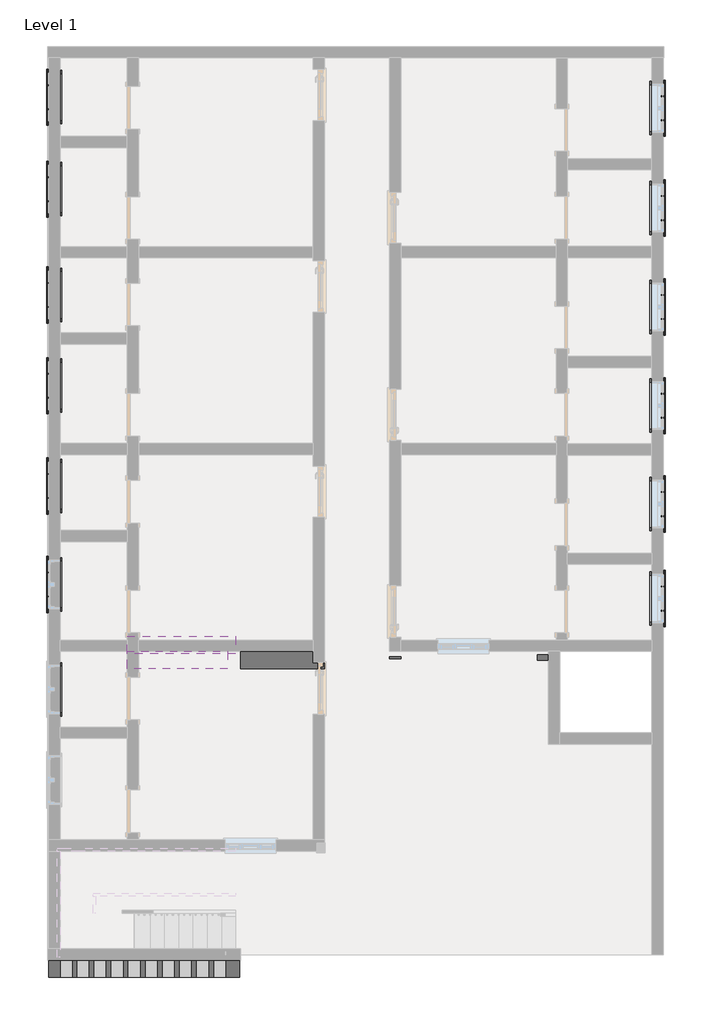
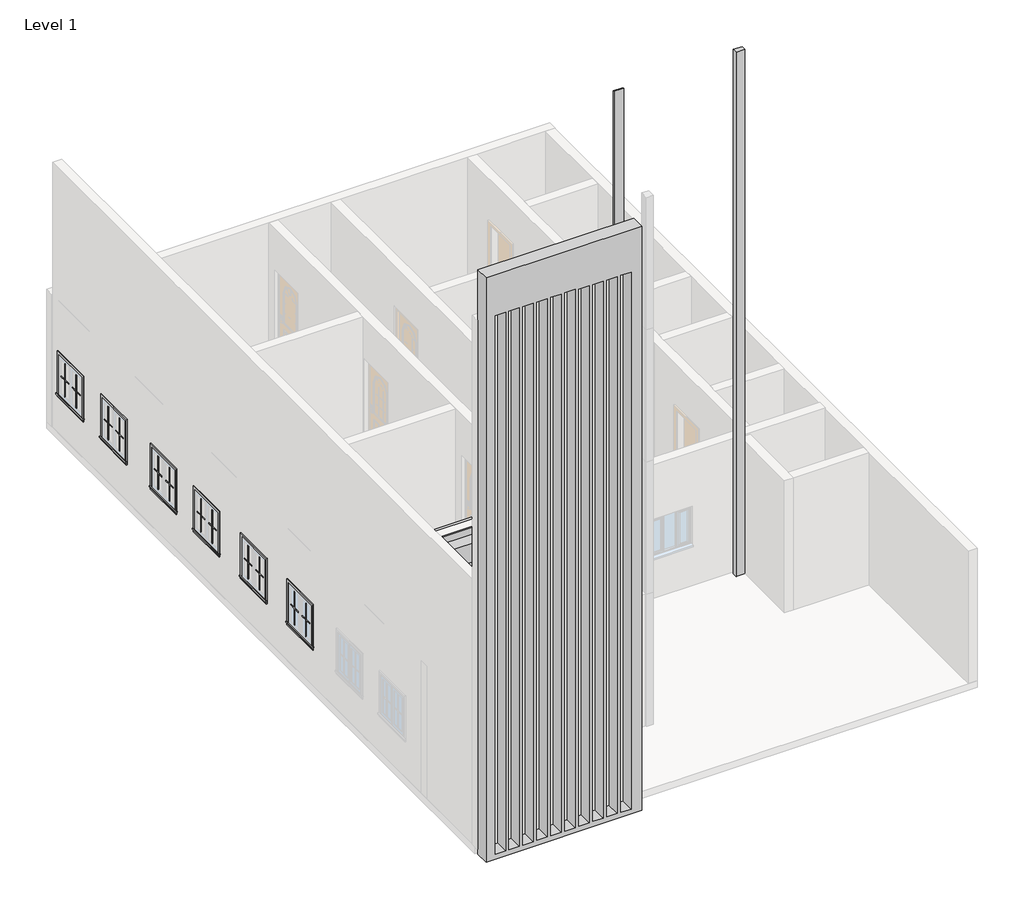
# One storey, part 4 of 4: 54 proxies.
"""IFC4 building model written with IfcOpenShell, lengths in millimetres."""

from ifc_helpers import new_model, si_unit, origin, place, context, project, spatial, transform, mapped, element, save
from components import generic_models_1_generic_models_1_2151a878, generic_models_2_generic_models_2_263b720d, generic_models_3_generic_models_3_38643fe6, generic_models_4_generic_models_4_c09d9ab6, generic_models_5_generic_models_5_710787d1, muntin_pattern_2x2_muntin_pattern_2x2_b3fe6957, muntin_pattern_2x2_muntin_pattern_2x2_3e0ecaf2, trim_window_exterior_flat_with_sill_41619996, trim_window_interior_flat_picture_frame_51c85655

model = new_model("IFC4")

# Units and contexts
model_context = context("Model", 3, world=origin())
ifc_project = project(units=[si_unit("LENGTHUNIT", "METRE", prefix="MILLI")], contexts=[model_context])

# Site, building, storey
site = spatial("IfcSite", under=ifc_project)
building = spatial("IfcBuilding", under=site)
storey = spatial("IfcBuildingStorey", under=building, Name="Level 1", Elevation=0.0)

# Proxies
placement = place(None, origin())
generic_models_1_generic_models_1_shape = generic_models_1_generic_models_1_2151a878(model_context)
element("IfcBuildingElementProxy", 1, Name="Generic Models 1 : Generic Models 1", ObjectType="Generic Models 1 : Generic Models 1", at=placement, inside=storey, context=model_context, shape_type="MappedRepresentation", body=[
    mapped(generic_models_1_generic_models_1_shape, transform((0.0, 0.0, 0.0), x_axis=(1.0, 0.0, 0.0), y_axis=(0.0, 1.0, 0.0), z_axis=(0.0, 0.0, 1.0))),
])
generic_models_2_generic_models_2_shape = generic_models_2_generic_models_2_263b720d(model_context)
element("IfcBuildingElementProxy", 2, Name="Generic Models 2 : Generic Models 2", ObjectType="Generic Models 2 : Generic Models 2", at=placement, inside=storey, context=model_context, shape_type="MappedRepresentation", body=[
    mapped(generic_models_2_generic_models_2_shape, transform((0.0, 0.0, 0.0), x_axis=(1.0, 0.0, 0.0), y_axis=(0.0, 1.0, 0.0), z_axis=(0.0, 0.0, 1.0))),
])
generic_models_3_generic_models_3_shape = generic_models_3_generic_models_3_38643fe6(model_context)
element("IfcBuildingElementProxy", 3, Name="Generic Models 3 : Generic Models 3", ObjectType="Generic Models 3 : Generic Models 3", at=placement, inside=storey, context=model_context, shape_type="MappedRepresentation", body=[
    mapped(generic_models_3_generic_models_3_shape, transform((0.0, 0.0, 0.0), x_axis=(1.0, 0.0, 0.0), y_axis=(0.0, 1.0, 0.0), z_axis=(0.0, 0.0, 1.0))),
])
generic_models_4_generic_models_4_shape = generic_models_4_generic_models_4_c09d9ab6(model_context)
element("IfcBuildingElementProxy", 4, Name="Generic Models 4 : Generic Models 4", ObjectType="Generic Models 4 : Generic Models 4", at=placement, inside=storey, context=model_context, shape_type="MappedRepresentation", body=[
    mapped(generic_models_4_generic_models_4_shape, transform((0.0, 0.0, 0.0), x_axis=(1.0, 0.0, 0.0), y_axis=(0.0, 1.0, 0.0), z_axis=(0.0, 0.0, 1.0))),
])
generic_models_5_generic_models_5_shape = generic_models_5_generic_models_5_710787d1(model_context)
element("IfcBuildingElementProxy", 5, Name="Generic Models 5 : Generic Models 5", ObjectType="Generic Models 5 : Generic Models 5", at=placement, inside=storey, context=model_context, shape_type="MappedRepresentation", body=[
    mapped(generic_models_5_generic_models_5_shape, transform((0.0, 0.0, 0.0), x_axis=(1.0, 0.0, 0.0), y_axis=(0.0, 1.0, 0.0), z_axis=(0.0, 0.0, 1.0))),
])
muntin_pattern_2x2_muntin_pattern_2x2_shape = muntin_pattern_2x2_muntin_pattern_2x2_b3fe6957(model_context)
element("IfcBuildingElementProxy", 6, Name="Muntin Pattern_2x2 : Muntin Pattern_2x2", ObjectType="Muntin Pattern_2x2 : Muntin Pattern_2x2", at=placement, inside=storey, context=model_context, shape_type="MappedRepresentation", body=[
    mapped(muntin_pattern_2x2_muntin_pattern_2x2_shape, transform((-6438.8858866, 6882.8274728, 984.25), x_axis=(0.0, 1.0, 0.0), y_axis=(-1.0, 0.0, 0.0), z_axis=(0.0, 0.0, 1.0))),
])
element("IfcBuildingElementProxy", 7, Name="Muntin Pattern_2x2 : Muntin Pattern_2x2", ObjectType="Muntin Pattern_2x2 : Muntin Pattern_2x2", at=placement, inside=storey, context=model_context, shape_type="MappedRepresentation", body=[
    mapped(muntin_pattern_2x2_muntin_pattern_2x2_shape, transform((-6438.8858866, 5244.5274728, 984.25), x_axis=(0.0, 1.0, 0.0), y_axis=(-1.0, 0.0, 0.0), z_axis=(0.0, 0.0, 1.0))),
])
element("IfcBuildingElementProxy", 8, Name="Muntin Pattern_2x2 : Muntin Pattern_2x2", ObjectType="Muntin Pattern_2x2 : Muntin Pattern_2x2", at=placement, inside=storey, context=model_context, shape_type="MappedRepresentation", body=[
    mapped(muntin_pattern_2x2_muntin_pattern_2x2_shape, transform((-6438.8858866, 3360.4810874, 984.25), x_axis=(0.0, 1.0, 0.0), y_axis=(-1.0, 0.0, 0.0), z_axis=(0.0, 0.0, 1.0))),
])
element("IfcBuildingElementProxy", 9, Name="Muntin Pattern_2x2 : Muntin Pattern_2x2", ObjectType="Muntin Pattern_2x2 : Muntin Pattern_2x2", at=placement, inside=storey, context=model_context, shape_type="MappedRepresentation", body=[
    mapped(muntin_pattern_2x2_muntin_pattern_2x2_shape, transform((-6438.8858866, 1745.426343, 984.25), x_axis=(0.0, 1.0, 0.0), y_axis=(-1.0, 0.0, 0.0), z_axis=(0.0, 0.0, 1.0))),
])
element("IfcBuildingElementProxy", 10, Name="Muntin Pattern_2x2 : Muntin Pattern_2x2", ObjectType="Muntin Pattern_2x2 : Muntin Pattern_2x2", at=placement, inside=storey, context=model_context, shape_type="MappedRepresentation", body=[
    mapped(muntin_pattern_2x2_muntin_pattern_2x2_shape, transform((-6438.8858866, -38.6725272, 984.25), x_axis=(0.0, 1.0, 0.0), y_axis=(-1.0, 0.0, 0.0), z_axis=(0.0, 0.0, 1.0))),
])
element("IfcBuildingElementProxy", 11, Name="Muntin Pattern_2x2 : Muntin Pattern_2x2", ObjectType="Muntin Pattern_2x2 : Muntin Pattern_2x2", at=placement, inside=storey, context=model_context, shape_type="MappedRepresentation", body=[
    mapped(muntin_pattern_2x2_muntin_pattern_2x2_shape, transform((-6438.8858866, -1791.2725272, 984.25), x_axis=(0.0, 1.0, 0.0), y_axis=(-1.0, 0.0, 0.0), z_axis=(0.0, 0.0, 1.0))),
])
element("IfcBuildingElementProxy", 12, Name="Muntin Pattern_2x2 : Muntin Pattern_2x2", ObjectType="Muntin Pattern_2x2 : Muntin Pattern_2x2", at=placement, inside=storey, context=model_context, shape_type="MappedRepresentation", body=[
    mapped(muntin_pattern_2x2_muntin_pattern_2x2_shape, transform((4489.4641134, -1616.6475272, 984.25), x_axis=(0.0, -1.0, 0.0), y_axis=(1.0, 0.0, 0.0), z_axis=(0.0, 0.0, 1.0))),
])
element("IfcBuildingElementProxy", 13, Name="Muntin Pattern_2x2 : Muntin Pattern_2x2", ObjectType="Muntin Pattern_2x2 : Muntin Pattern_2x2", at=placement, inside=storey, context=model_context, shape_type="MappedRepresentation", body=[
    mapped(muntin_pattern_2x2_muntin_pattern_2x2_shape, transform((4489.4641134, 66.1024728, 984.25), x_axis=(0.0, -1.0, 0.0), y_axis=(1.0, 0.0, 0.0), z_axis=(0.0, 0.0, 1.0))),
])
element("IfcBuildingElementProxy", 14, Name="Muntin Pattern_2x2 : Muntin Pattern_2x2", ObjectType="Muntin Pattern_2x2 : Muntin Pattern_2x2", at=placement, inside=storey, context=model_context, shape_type="MappedRepresentation", body=[
    mapped(muntin_pattern_2x2_muntin_pattern_2x2_shape, transform((4489.4641134, 1818.7024728, 984.25), x_axis=(0.0, -1.0, 0.0), y_axis=(1.0, 0.0, 0.0), z_axis=(0.0, 0.0, 1.0))),
])
element("IfcBuildingElementProxy", 15, Name="Muntin Pattern_2x2 : Muntin Pattern_2x2", ObjectType="Muntin Pattern_2x2 : Muntin Pattern_2x2", at=placement, inside=storey, context=model_context, shape_type="MappedRepresentation", body=[
    mapped(muntin_pattern_2x2_muntin_pattern_2x2_shape, transform((4489.4641134, 3577.6524728, 984.25), x_axis=(0.0, -1.0, 0.0), y_axis=(1.0, 0.0, 0.0), z_axis=(0.0, 0.0, 1.0))),
])
element("IfcBuildingElementProxy", 16, Name="Muntin Pattern_2x2 : Muntin Pattern_2x2", ObjectType="Muntin Pattern_2x2 : Muntin Pattern_2x2", at=placement, inside=storey, context=model_context, shape_type="MappedRepresentation", body=[
    mapped(muntin_pattern_2x2_muntin_pattern_2x2_shape, transform((4489.4641134, 5336.6024728, 984.25), x_axis=(0.0, -1.0, 0.0), y_axis=(1.0, 0.0, 0.0), z_axis=(0.0, 0.0, 1.0))),
])
element("IfcBuildingElementProxy", 17, Name="Muntin Pattern_2x2 : Muntin Pattern_2x2", ObjectType="Muntin Pattern_2x2 : Muntin Pattern_2x2", at=placement, inside=storey, context=model_context, shape_type="MappedRepresentation", body=[
    mapped(muntin_pattern_2x2_muntin_pattern_2x2_shape, transform((4489.4641134, 7114.6024728, 984.25), x_axis=(0.0, -1.0, 0.0), y_axis=(1.0, 0.0, 0.0), z_axis=(0.0, 0.0, 1.0))),
])
muntin_pattern_2x2_muntin_pattern_2x2_2_shape = muntin_pattern_2x2_muntin_pattern_2x2_3e0ecaf2(model_context)
element("IfcBuildingElementProxy", 18, Name="Muntin Pattern_2x2 : Muntin Pattern_2x2", ObjectType="Muntin Pattern_2x2 : Muntin Pattern_2x2", at=placement, inside=storey, context=model_context, shape_type="MappedRepresentation", body=[
    mapped(muntin_pattern_2x2_muntin_pattern_2x2_2_shape, transform((-6438.8858866, 7311.4524728, 984.25), x_axis=(0.0, -1.0, 0.0), y_axis=(1.0, 0.0, 0.0), z_axis=(0.0, 0.0, 1.0))),
])
element("IfcBuildingElementProxy", 19, Name="Muntin Pattern_2x2 : Muntin Pattern_2x2", ObjectType="Muntin Pattern_2x2 : Muntin Pattern_2x2", at=placement, inside=storey, context=model_context, shape_type="MappedRepresentation", body=[
    mapped(muntin_pattern_2x2_muntin_pattern_2x2_2_shape, transform((-6438.8858866, 5673.1524728, 984.25), x_axis=(0.0, -1.0, 0.0), y_axis=(1.0, 0.0, 0.0), z_axis=(0.0, 0.0, 1.0))),
])
element("IfcBuildingElementProxy", 20, Name="Muntin Pattern_2x2 : Muntin Pattern_2x2", ObjectType="Muntin Pattern_2x2 : Muntin Pattern_2x2", at=placement, inside=storey, context=model_context, shape_type="MappedRepresentation", body=[
    mapped(muntin_pattern_2x2_muntin_pattern_2x2_2_shape, transform((-6438.8858866, 3789.1060874, 984.25), x_axis=(0.0, -1.0, 0.0), y_axis=(1.0, 0.0, 0.0), z_axis=(0.0, 0.0, 1.0))),
])
element("IfcBuildingElementProxy", 21, Name="Muntin Pattern_2x2 : Muntin Pattern_2x2", ObjectType="Muntin Pattern_2x2 : Muntin Pattern_2x2", at=placement, inside=storey, context=model_context, shape_type="MappedRepresentation", body=[
    mapped(muntin_pattern_2x2_muntin_pattern_2x2_2_shape, transform((-6438.8858866, 2174.051343, 984.25), x_axis=(0.0, -1.0, 0.0), y_axis=(1.0, 0.0, 0.0), z_axis=(0.0, 0.0, 1.0))),
])
element("IfcBuildingElementProxy", 22, Name="Muntin Pattern_2x2 : Muntin Pattern_2x2", ObjectType="Muntin Pattern_2x2 : Muntin Pattern_2x2", at=placement, inside=storey, context=model_context, shape_type="MappedRepresentation", body=[
    mapped(muntin_pattern_2x2_muntin_pattern_2x2_2_shape, transform((-6438.8858866, 389.9524728, 984.25), x_axis=(0.0, -1.0, 0.0), y_axis=(1.0, 0.0, 0.0), z_axis=(0.0, 0.0, 1.0))),
])
element("IfcBuildingElementProxy", 23, Name="Muntin Pattern_2x2 : Muntin Pattern_2x2", ObjectType="Muntin Pattern_2x2 : Muntin Pattern_2x2", at=placement, inside=storey, context=model_context, shape_type="MappedRepresentation", body=[
    mapped(muntin_pattern_2x2_muntin_pattern_2x2_2_shape, transform((-6438.8858866, -1362.6475272, 984.25), x_axis=(0.0, -1.0, 0.0), y_axis=(1.0, 0.0, 0.0), z_axis=(0.0, 0.0, 1.0))),
])
element("IfcBuildingElementProxy", 24, Name="Muntin Pattern_2x2 : Muntin Pattern_2x2", ObjectType="Muntin Pattern_2x2 : Muntin Pattern_2x2", at=placement, inside=storey, context=model_context, shape_type="MappedRepresentation", body=[
    mapped(muntin_pattern_2x2_muntin_pattern_2x2_2_shape, transform((4489.4641134, -2045.2725272, 984.25), x_axis=(0.0, 1.0, 0.0), y_axis=(-1.0, 0.0, 0.0), z_axis=(0.0, 0.0, 1.0))),
])
element("IfcBuildingElementProxy", 25, Name="Muntin Pattern_2x2 : Muntin Pattern_2x2", ObjectType="Muntin Pattern_2x2 : Muntin Pattern_2x2", at=placement, inside=storey, context=model_context, shape_type="MappedRepresentation", body=[
    mapped(muntin_pattern_2x2_muntin_pattern_2x2_2_shape, transform((4489.4641134, -362.5225272, 984.25), x_axis=(0.0, 1.0, 0.0), y_axis=(-1.0, 0.0, 0.0), z_axis=(0.0, 0.0, 1.0))),
])
element("IfcBuildingElementProxy", 26, Name="Muntin Pattern_2x2 : Muntin Pattern_2x2", ObjectType="Muntin Pattern_2x2 : Muntin Pattern_2x2", at=placement, inside=storey, context=model_context, shape_type="MappedRepresentation", body=[
    mapped(muntin_pattern_2x2_muntin_pattern_2x2_2_shape, transform((4489.4641134, 1390.0774728, 984.25), x_axis=(0.0, 1.0, 0.0), y_axis=(-1.0, 0.0, 0.0), z_axis=(0.0, 0.0, 1.0))),
])
element("IfcBuildingElementProxy", 27, Name="Muntin Pattern_2x2 : Muntin Pattern_2x2", ObjectType="Muntin Pattern_2x2 : Muntin Pattern_2x2", at=placement, inside=storey, context=model_context, shape_type="MappedRepresentation", body=[
    mapped(muntin_pattern_2x2_muntin_pattern_2x2_2_shape, transform((4489.4641134, 3149.0274728, 984.25), x_axis=(0.0, 1.0, 0.0), y_axis=(-1.0, 0.0, 0.0), z_axis=(0.0, 0.0, 1.0))),
])
element("IfcBuildingElementProxy", 28, Name="Muntin Pattern_2x2 : Muntin Pattern_2x2", ObjectType="Muntin Pattern_2x2 : Muntin Pattern_2x2", at=placement, inside=storey, context=model_context, shape_type="MappedRepresentation", body=[
    mapped(muntin_pattern_2x2_muntin_pattern_2x2_2_shape, transform((4489.4641134, 4907.9774728, 984.25), x_axis=(0.0, 1.0, 0.0), y_axis=(-1.0, 0.0, 0.0), z_axis=(0.0, 0.0, 1.0))),
])
element("IfcBuildingElementProxy", 29, Name="Muntin Pattern_2x2 : Muntin Pattern_2x2", ObjectType="Muntin Pattern_2x2 : Muntin Pattern_2x2", at=placement, inside=storey, context=model_context, shape_type="MappedRepresentation", body=[
    mapped(muntin_pattern_2x2_muntin_pattern_2x2_2_shape, transform((4489.4641134, 6685.9774728, 984.25), x_axis=(0.0, 1.0, 0.0), y_axis=(-1.0, 0.0, 0.0), z_axis=(0.0, 0.0, 1.0))),
])
trim_window_exterior_flat_with_sill_shape = trim_window_exterior_flat_with_sill_41619996(model_context)
element("IfcBuildingElementProxy", 30, Name="Trim-Window-Exterior-Flat : with Sill", ObjectType="Trim-Window-Exterior-Flat : with Sill", at=placement, inside=storey, context=model_context, shape_type="MappedRepresentation", body=[
    mapped(trim_window_exterior_flat_with_sill_shape, transform((-6448.4108866, 7097.1399728, 1828.8), x_axis=(0.0, -1.0, 0.0), y_axis=(0.0, 0.0, 1.0), z_axis=(-1.0, 0.0, 0.0))),
])
element("IfcBuildingElementProxy", 31, Name="Trim-Window-Exterior-Flat : with Sill", ObjectType="Trim-Window-Exterior-Flat : with Sill", at=placement, inside=storey, context=model_context, shape_type="MappedRepresentation", body=[
    mapped(trim_window_exterior_flat_with_sill_shape, transform((-6448.4108866, 5458.8399728, 1828.8), x_axis=(0.0, -1.0, 0.0), y_axis=(0.0, 0.0, 1.0), z_axis=(-1.0, 0.0, 0.0))),
])
element("IfcBuildingElementProxy", 32, Name="Trim-Window-Exterior-Flat : with Sill", ObjectType="Trim-Window-Exterior-Flat : with Sill", at=placement, inside=storey, context=model_context, shape_type="MappedRepresentation", body=[
    mapped(trim_window_exterior_flat_with_sill_shape, transform((-6448.4108866, 3574.7935874, 1828.8), x_axis=(0.0, -1.0, 0.0), y_axis=(0.0, 0.0, 1.0), z_axis=(-1.0, 0.0, 0.0))),
])
element("IfcBuildingElementProxy", 33, Name="Trim-Window-Exterior-Flat : with Sill", ObjectType="Trim-Window-Exterior-Flat : with Sill", at=placement, inside=storey, context=model_context, shape_type="MappedRepresentation", body=[
    mapped(trim_window_exterior_flat_with_sill_shape, transform((-6448.4108866, 1959.738843, 1828.8), x_axis=(0.0, -1.0, 0.0), y_axis=(0.0, 0.0, 1.0), z_axis=(-1.0, 0.0, 0.0))),
])
element("IfcBuildingElementProxy", 34, Name="Trim-Window-Exterior-Flat : with Sill", ObjectType="Trim-Window-Exterior-Flat : with Sill", at=placement, inside=storey, context=model_context, shape_type="MappedRepresentation", body=[
    mapped(trim_window_exterior_flat_with_sill_shape, transform((-6448.4108866, 175.6399728, 1828.8), x_axis=(0.0, -1.0, 0.0), y_axis=(0.0, 0.0, 1.0), z_axis=(-1.0, 0.0, 0.0))),
])
element("IfcBuildingElementProxy", 35, Name="Trim-Window-Exterior-Flat : with Sill", ObjectType="Trim-Window-Exterior-Flat : with Sill", at=placement, inside=storey, context=model_context, shape_type="MappedRepresentation", body=[
    mapped(trim_window_exterior_flat_with_sill_shape, transform((-6448.4108866, -1576.9600272, 1828.8), x_axis=(0.0, -1.0, 0.0), y_axis=(0.0, 0.0, 1.0), z_axis=(-1.0, 0.0, 0.0))),
])
element("IfcBuildingElementProxy", 36, Name="Trim-Window-Exterior-Flat : with Sill", ObjectType="Trim-Window-Exterior-Flat : with Sill", at=placement, inside=storey, context=model_context, shape_type="MappedRepresentation", body=[
    mapped(trim_window_exterior_flat_with_sill_shape, transform((4498.9891134, -1830.9600272, 1828.8), x_axis=(0.0, 1.0, 0.0), y_axis=(0.0, 0.0, 1.0), z_axis=(1.0, 0.0, 0.0))),
])
element("IfcBuildingElementProxy", 37, Name="Trim-Window-Exterior-Flat : with Sill", ObjectType="Trim-Window-Exterior-Flat : with Sill", at=placement, inside=storey, context=model_context, shape_type="MappedRepresentation", body=[
    mapped(trim_window_exterior_flat_with_sill_shape, transform((4498.9891134, -148.2100272, 1828.8), x_axis=(0.0, 1.0, 0.0), y_axis=(0.0, 0.0, 1.0), z_axis=(1.0, 0.0, 0.0))),
])
element("IfcBuildingElementProxy", 38, Name="Trim-Window-Exterior-Flat : with Sill", ObjectType="Trim-Window-Exterior-Flat : with Sill", at=placement, inside=storey, context=model_context, shape_type="MappedRepresentation", body=[
    mapped(trim_window_exterior_flat_with_sill_shape, transform((4498.9891134, 1604.3899728, 1828.8), x_axis=(0.0, 1.0, 0.0), y_axis=(0.0, 0.0, 1.0), z_axis=(1.0, 0.0, 0.0))),
])
element("IfcBuildingElementProxy", 39, Name="Trim-Window-Exterior-Flat : with Sill", ObjectType="Trim-Window-Exterior-Flat : with Sill", at=placement, inside=storey, context=model_context, shape_type="MappedRepresentation", body=[
    mapped(trim_window_exterior_flat_with_sill_shape, transform((4498.9891134, 3363.3399728, 1828.8), x_axis=(0.0, 1.0, 0.0), y_axis=(0.0, 0.0, 1.0), z_axis=(1.0, 0.0, 0.0))),
])
element("IfcBuildingElementProxy", 40, Name="Trim-Window-Exterior-Flat : with Sill", ObjectType="Trim-Window-Exterior-Flat : with Sill", at=placement, inside=storey, context=model_context, shape_type="MappedRepresentation", body=[
    mapped(trim_window_exterior_flat_with_sill_shape, transform((4498.9891134, 5122.2899728, 1828.8), x_axis=(0.0, 1.0, 0.0), y_axis=(0.0, 0.0, 1.0), z_axis=(1.0, 0.0, 0.0))),
])
element("IfcBuildingElementProxy", 41, Name="Trim-Window-Exterior-Flat : with Sill", ObjectType="Trim-Window-Exterior-Flat : with Sill", at=placement, inside=storey, context=model_context, shape_type="MappedRepresentation", body=[
    mapped(trim_window_exterior_flat_with_sill_shape, transform((4498.9891134, 6900.2899728, 1828.8), x_axis=(0.0, 1.0, 0.0), y_axis=(0.0, 0.0, 1.0), z_axis=(1.0, 0.0, 0.0))),
])
trim_window_interior_flat_picture_frame_shape = trim_window_interior_flat_picture_frame_51c85655(model_context)
element("IfcBuildingElementProxy", 42, Name="Trim-Window-Interior-Flat : Picture Frame", ObjectType="Trim-Window-Interior-Flat : Picture Frame", at=placement, inside=storey, context=model_context, shape_type="MappedRepresentation", body=[
    mapped(trim_window_interior_flat_picture_frame_shape, transform((-6245.2108866, 7097.1399728, 1828.8), x_axis=(0.0, 1.0, 0.0), y_axis=(0.0, 0.0, 1.0), z_axis=(1.0, 0.0, 0.0))),
])
element("IfcBuildingElementProxy", 43, Name="Trim-Window-Interior-Flat : Picture Frame", ObjectType="Trim-Window-Interior-Flat : Picture Frame", at=placement, inside=storey, context=model_context, shape_type="MappedRepresentation", body=[
    mapped(trim_window_interior_flat_picture_frame_shape, transform((-6245.2108866, 5458.8399728, 1828.8), x_axis=(0.0, 1.0, 0.0), y_axis=(0.0, 0.0, 1.0), z_axis=(1.0, 0.0, 0.0))),
])
element("IfcBuildingElementProxy", 44, Name="Trim-Window-Interior-Flat : Picture Frame", ObjectType="Trim-Window-Interior-Flat : Picture Frame", at=placement, inside=storey, context=model_context, shape_type="MappedRepresentation", body=[
    mapped(trim_window_interior_flat_picture_frame_shape, transform((-6245.2108866, 3574.7935874, 1828.8), x_axis=(0.0, 1.0, 0.0), y_axis=(0.0, 0.0, 1.0), z_axis=(1.0, 0.0, 0.0))),
])
element("IfcBuildingElementProxy", 45, Name="Trim-Window-Interior-Flat : Picture Frame", ObjectType="Trim-Window-Interior-Flat : Picture Frame", at=placement, inside=storey, context=model_context, shape_type="MappedRepresentation", body=[
    mapped(trim_window_interior_flat_picture_frame_shape, transform((-6245.2108866, 1959.738843, 1828.8), x_axis=(0.0, 1.0, 0.0), y_axis=(0.0, 0.0, 1.0), z_axis=(1.0, 0.0, 0.0))),
])
element("IfcBuildingElementProxy", 46, Name="Trim-Window-Interior-Flat : Picture Frame", ObjectType="Trim-Window-Interior-Flat : Picture Frame", at=placement, inside=storey, context=model_context, shape_type="MappedRepresentation", body=[
    mapped(trim_window_interior_flat_picture_frame_shape, transform((-6245.2108866, 175.6399728, 1828.8), x_axis=(0.0, 1.0, 0.0), y_axis=(0.0, 0.0, 1.0), z_axis=(1.0, 0.0, 0.0))),
])
element("IfcBuildingElementProxy", 47, Name="Trim-Window-Interior-Flat : Picture Frame", ObjectType="Trim-Window-Interior-Flat : Picture Frame", at=placement, inside=storey, context=model_context, shape_type="MappedRepresentation", body=[
    mapped(trim_window_interior_flat_picture_frame_shape, transform((-6245.2108866, -1576.9600272, 1828.8), x_axis=(0.0, 1.0, 0.0), y_axis=(0.0, 0.0, 1.0), z_axis=(1.0, 0.0, 0.0))),
])
element("IfcBuildingElementProxy", 48, Name="Trim-Window-Interior-Flat : Picture Frame", ObjectType="Trim-Window-Interior-Flat : Picture Frame", at=placement, inside=storey, context=model_context, shape_type="MappedRepresentation", body=[
    mapped(trim_window_interior_flat_picture_frame_shape, transform((-6245.2108866, -3443.8600272, 1828.8), x_axis=(0.0, 1.0, 0.0), y_axis=(0.0, 0.0, 1.0), z_axis=(1.0, 0.0, 0.0))),
])
element("IfcBuildingElementProxy", 49, Name="Trim-Window-Interior-Flat : Picture Frame", ObjectType="Trim-Window-Interior-Flat : Picture Frame", at=placement, inside=storey, context=model_context, shape_type="MappedRepresentation", body=[
    mapped(trim_window_interior_flat_picture_frame_shape, transform((4295.7891134, -1830.9600272, 1828.8), x_axis=(0.0, -1.0, 0.0), y_axis=(0.0, 0.0, 1.0), z_axis=(-1.0, 0.0, 0.0))),
])
element("IfcBuildingElementProxy", 50, Name="Trim-Window-Interior-Flat : Picture Frame", ObjectType="Trim-Window-Interior-Flat : Picture Frame", at=placement, inside=storey, context=model_context, shape_type="MappedRepresentation", body=[
    mapped(trim_window_interior_flat_picture_frame_shape, transform((4295.7891134, -148.2100272, 1828.8), x_axis=(0.0, -1.0, 0.0), y_axis=(0.0, 0.0, 1.0), z_axis=(-1.0, 0.0, 0.0))),
])
element("IfcBuildingElementProxy", 51, Name="Trim-Window-Interior-Flat : Picture Frame", ObjectType="Trim-Window-Interior-Flat : Picture Frame", at=placement, inside=storey, context=model_context, shape_type="MappedRepresentation", body=[
    mapped(trim_window_interior_flat_picture_frame_shape, transform((4295.7891134, 1604.3899728, 1828.8), x_axis=(0.0, -1.0, 0.0), y_axis=(0.0, 0.0, 1.0), z_axis=(-1.0, 0.0, 0.0))),
])
element("IfcBuildingElementProxy", 52, Name="Trim-Window-Interior-Flat : Picture Frame", ObjectType="Trim-Window-Interior-Flat : Picture Frame", at=placement, inside=storey, context=model_context, shape_type="MappedRepresentation", body=[
    mapped(trim_window_interior_flat_picture_frame_shape, transform((4295.7891134, 3363.3399728, 1828.8), x_axis=(0.0, -1.0, 0.0), y_axis=(0.0, 0.0, 1.0), z_axis=(-1.0, 0.0, 0.0))),
])
element("IfcBuildingElementProxy", 53, Name="Trim-Window-Interior-Flat : Picture Frame", ObjectType="Trim-Window-Interior-Flat : Picture Frame", at=placement, inside=storey, context=model_context, shape_type="MappedRepresentation", body=[
    mapped(trim_window_interior_flat_picture_frame_shape, transform((4295.7891134, 5122.2899728, 1828.8), x_axis=(0.0, -1.0, 0.0), y_axis=(0.0, 0.0, 1.0), z_axis=(-1.0, 0.0, 0.0))),
])
element("IfcBuildingElementProxy", 54, Name="Trim-Window-Interior-Flat : Picture Frame", ObjectType="Trim-Window-Interior-Flat : Picture Frame", at=placement, inside=storey, context=model_context, shape_type="MappedRepresentation", body=[
    mapped(trim_window_interior_flat_picture_frame_shape, transform((4295.7891134, 6900.2899728, 1828.8), x_axis=(0.0, -1.0, 0.0), y_axis=(0.0, 0.0, 1.0), z_axis=(-1.0, 0.0, 0.0))),
])

save(model, "model.ifc")

# Revit data of these elements
# Type "Muntin Pattern_2x2 : Muntin Pattern_2x2"
#   Width [instance default] = 4' - 0"
#   Thickness = 0' - 0 1/2"
#   Height [instance default] = 4' - 0"
#   Distance = 0' - 0 3/4"
#   Interior Material [instance default] = none
#   Exterior Material [instance default] = none
#   Default Elevation = 0
# Type "Trim-Window-Exterior-Flat : with Sill"
#   Trim Width = 0' - 2 1/4"
#   Trim Thickness_Picture Frame = 0' - 1 1/4"
#   Trim Thickness_with Sill = 0' - 0 3/4"
#   Sill Thickness = 0' - 1 1/4"
#   Opening Width [instance default] = 2' - 0"
#   Opening Height [instance default] = 3' - 0"
#   Default Elevation = 4' - 0"
#   Sill = yes
#   Picture Frame = no
#   Trim Material [instance default] = none
# Type "Trim-Window-Interior-Flat : Picture Frame"
#   Trim Thickness_Picture Frame = 0' - 1 1/4"
#   Trim Width = 0' - 2 1/4"
#   Trim Thickness_with Sill = 0' - 0 3/4"
#   Sill Thickness = 0' - 1 1/4"
#   Opening Width [instance default] = 2' - 0"
#   Opening Height [instance default] = 3' - 0"
#   Default Elevation = 4' - 0"
#   Sill = no
#   Picture Frame = yes
#   Trim Material [instance default] = none
# Element 1 (IfcBuildingElementProxy, "Generic Models 1 : Generic Models 1")
#   Phase Created = New Construction
#   Materials on its faces: "Doors - Glazing Bars", "Earth"
# Element 2 (IfcBuildingElementProxy, "Generic Models 2 : Generic Models 2")
#   Phase Created = New Construction
# Element 3 (IfcBuildingElementProxy, "Generic Models 3 : Generic Models 3")
#   Phase Created = New Construction
# Element 4 (IfcBuildingElementProxy, "Generic Models 4 : Generic Models 4")
#   Phase Created = New Construction
#   Materials on its faces: "Oak Flooring", "Window Frame"
# Element 5 (IfcBuildingElementProxy, "Generic Models 5 : Generic Models 5")
#   Phase Created = New Construction
# Elements 6, 7, 8, 9, 10, 11, 12, 13, 14, 15, 16, 17, 18, 19, 20, 21, 22, 23, 24, 25, 26, 27, 28, 29 (IfcBuildingElementProxy, "Muntin Pattern_2x2 : Muntin Pattern_2x2")
#   Width = 0' - 11 5/8"
#   Height = 2' - 6 1/2"
#   Interior Material = Wood - Stained
#   Exterior Material = Clad - White
#   Phase Created = New Construction
#   Materials on its faces: "Clad - White", "Wood - Stained"
# Elements 30, 31, 32, 33, 34, 35, 36, 37, 38, 39, 40, 41 (IfcBuildingElementProxy, "Trim-Window-Exterior-Flat : with Sill")
#   Opening Width = 2' - 10"
#   Opening Height = 3' - 0"
#   Trim Material = Clad - White
#   Phase Created = New Construction
#   Materials on its faces: "Clad - White"
# Elements 42, 43, 44, 45, 46, 47, 48, 49, 50, 51, 52, 53, 54 (IfcBuildingElementProxy, "Trim-Window-Interior-Flat : Picture Frame")
#   Opening Width = 2' - 10"
#   Opening Height = 3' - 0"
#   Trim Material = Wood - Stained
#   Phase Created = New Construction
#   Materials on its faces: "Wood - Stained"
# Materials
#   "Doors - Glazing Bars": colour RGB 158 107 65, transparency 0
#   "Earth": class "Generic", colour RGB 97 75 62, transparency 0, Description = "Soil", Cost = 0
#   "Oak Flooring": class "Wood", colour RGB 216 169 114, transparency 0, Description = "Quercus Rubra", Cost = 0
#   "Window Frame": colour RGB 249 249 249, transparency 0
#   "Clad - White": class "Wood", colour RGB 242 242 238, transparency 0, Cost = 0
#   "Wood - Stained": class "Wood", colour RGB 224 178 126, transparency 0, Cost = 0
